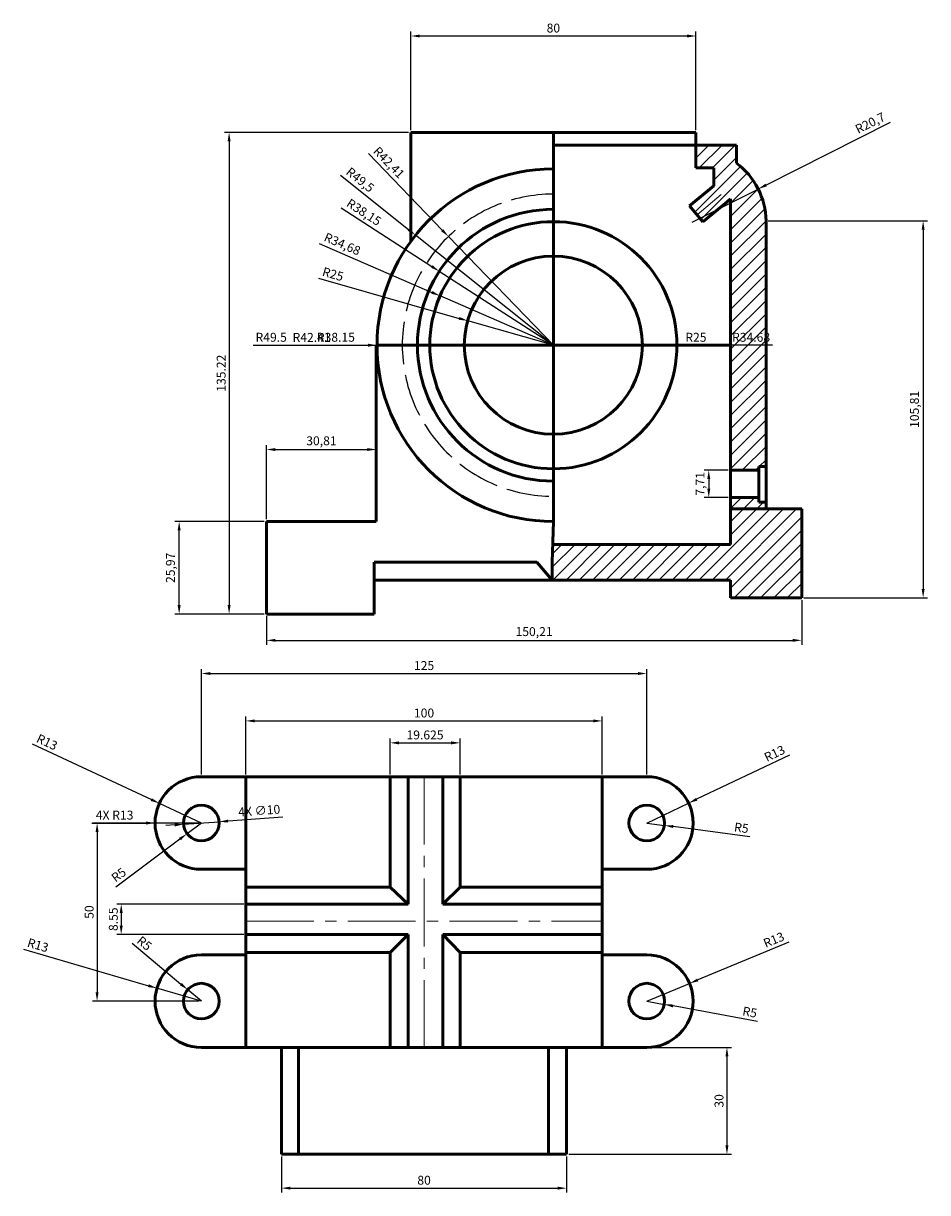
# Model space of a CAD drawing. Units: millimetres. Extents: x 1140 to 1880, y 1480 to 1815.
# Tile 3 of 3: x 1626 to 1880, y 1487 to 1815. Entities that reach past the tile are written whole.
import ezdxf

# ---------------------------------------------------------------- set-up
doc = ezdxf.new("R2010")
doc.units = ezdxf.units.MM
doc.linetypes.add('ACAD_ISO02W100', pattern=[15, 12, -3])
doc.linetypes.add('CENTER2', pattern=[28.575, 19.05, -3.175, 3.175, -3.175])
for name, color, linetype, lineweight in [('M-CNTR', 1, 'CENTER2', 18), ('M-DIMS', 2, 'Continuous', 25), ('M-HATC', 8, 'Continuous', 18), ('M-HIDN', 6, 'ACAD_ISO02W100', 25), ('M-OUTL', 7, 'Continuous', 50)]:
    doc.layers.add(name, color=color, linetype=linetype, lineweight=lineweight)
doc.styles.get("Standard").update_dxf_attribs({"font": 'arial.ttf'})
doc.dimstyles.new('ISO-25', dxfattribs={"dimtxt": 2.5, "dimasz": 2.5, "dimexe": 1.25, "dimexo": 0.625, "dimtad": 1, "dimtxsty": 'Standard', "dimcen": 2.5, "dimadec": 0, "dimazin": 0, "dimtfac": 1, "dimtmove": 0, "dimatfit": 3, "dimfxl": 1, "dimarcsym": 0})

# ---------------------------------------------------------------- blocks, each defined once
blk = doc.blocks.new('*D58')
at = {"layer": 'Defpoints', "color": 0, "transparency": 16777216}
for p in [(1788.55, 1619.58), (1688.55, 1603.92), (1788.55, 1603.92)]:
    blk.add_point(p, dxfattribs=at)
at = {"layer": 'M-DIMS', "color": 0, "lineweight": -2, "transparency": 16777216}
for p, q in [((1688.55, 1604.54), (1688.55, 1620.83)), ((1691.05, 1619.58), (1786.05, 1619.58)), ((1788.55, 1604.54), (1788.55, 1620.83))]:
    blk.add_line(p, q, dxfattribs=at)
at = {"layer": 'M-DIMS', "color": 0, "transparency": 16777216}
for points in [[(1691.05, 1620), (1691.05, 1619.16), (1688.55, 1619.58)], [(1786.05, 1620), (1786.05, 1619.16), (1788.55, 1619.58)]]:
    blk.add_solid(points, dxfattribs=at)
at = {"layer": 'M-DIMS', "color": 0, "transparency": 16777216, "insert": (1738.55, 1621.48), "char_height": 2.5, "attachment_point": 5}
blk.add_mtext('100', dxfattribs=at)
blk = doc.blocks.new('*D59')
at = {"layer": 'Defpoints', "color": 0, "transparency": 16777216}
for p in [(1801.05, 1632.89), (1676.05, 1603.92), (1801.05, 1603.92)]:
    blk.add_point(p, dxfattribs=at)
at = {"layer": 'M-DIMS', "color": 0, "lineweight": -2, "transparency": 16777216}
for p, q in [((1676.05, 1604.54), (1676.05, 1634.14)), ((1678.55, 1632.89), (1798.55, 1632.89)), ((1801.05, 1604.54), (1801.05, 1634.14))]:
    blk.add_line(p, q, dxfattribs=at)
at = {"layer": 'M-DIMS', "color": 0, "transparency": 16777216}
for points in [[(1678.55, 1633.3), (1678.55, 1632.47), (1676.05, 1632.89)], [(1798.55, 1633.3), (1798.55, 1632.47), (1801.05, 1632.89)]]:
    blk.add_solid(points, dxfattribs=at)
at = {"layer": 'M-DIMS', "color": 0, "transparency": 16777216, "insert": (1738.55, 1634.79), "char_height": 2.5, "attachment_point": 5}
blk.add_mtext('125', dxfattribs=at)
blk = doc.blocks.new('*D60')
at = {"layer": 'Defpoints', "color": 0, "transparency": 16777216}
for p in [(1676.05, 1590.92), (1646.78, 1540.92), (1676.05, 1540.92)]:
    blk.add_point(p, dxfattribs=at)
at = {"layer": 'M-DIMS', "color": 0, "lineweight": -2, "transparency": 16777216}
for p, q in [((1675.42, 1590.92), (1645.53, 1590.92)), ((1646.78, 1588.42), (1646.78, 1543.42)), ((1675.42, 1540.92), (1645.53, 1540.92))]:
    blk.add_line(p, q, dxfattribs=at)
at = {"layer": 'M-DIMS', "color": 0, "transparency": 16777216}
for points in [[(1646.36, 1588.42), (1647.19, 1588.42), (1646.78, 1590.92)], [(1646.36, 1543.42), (1647.19, 1543.42), (1646.78, 1540.92)]]:
    blk.add_solid(points, dxfattribs=at)
at = {"layer": 'M-DIMS', "color": 0, "transparency": 16777216, "insert": (1644.88, 1565.92), "char_height": 2.5, "attachment_point": 5, "rotation": 90}
blk.add_mtext('50', dxfattribs=at)
blk = doc.blocks.new('*D61')
at = {"layer": 'Defpoints', "color": 0, "transparency": 16777216}
for p in [(1812.79, 1596.5), (1801.05, 1590.92)]:
    blk.add_point(p, dxfattribs=at)
at = {"layer": 'M-DIMS', "color": 0, "lineweight": -2, "transparency": 16777216}
for p, q in [((1841.13, 1609.99), (1815.05, 1597.58)), ((1801.05, 1590.92), (1812.79, 1596.5))]:
    blk.add_line(p, q, dxfattribs=at)
at = {"layer": 'M-DIMS', "color": 0, "transparency": 16777216}
blk.add_solid([(1814.87, 1597.95), (1815.22, 1597.2), (1812.79, 1596.5)], dxfattribs=at)
at = {"layer": 'M-DIMS', "color": 0, "transparency": 16777216, "insert": (1837.05, 1610.16), "char_height": 2.5, "attachment_point": 5, "rotation": 25.4449}
blk.add_mtext('R13', dxfattribs=at)
blk = doc.blocks.new('*D62')
at = {"layer": 'Defpoints', "color": 0, "transparency": 16777216}
for p in [(1813.05, 1545.91), (1801.05, 1540.92)]:
    blk.add_point(p, dxfattribs=at)
at = {"layer": 'M-DIMS', "color": 0, "lineweight": -2, "transparency": 16777216}
for p, q in [((1840.89, 1557.47), (1815.36, 1546.87)), ((1801.05, 1540.92), (1813.05, 1545.91))]:
    blk.add_line(p, q, dxfattribs=at)
at = {"layer": 'M-DIMS', "color": 0, "transparency": 16777216}
blk.add_solid([(1815.2, 1547.25), (1815.52, 1546.48), (1813.05, 1545.91)], dxfattribs=at)
at = {"layer": 'M-DIMS', "color": 0, "transparency": 16777216, "insert": (1836.82, 1557.84), "char_height": 2.5, "attachment_point": 5, "rotation": 22.5655}
blk.add_mtext('R13', dxfattribs=at)
blk = doc.blocks.new('*D63')
at = {"layer": 'Defpoints', "color": 0, "transparency": 16777216}
for p in [(1663.57, 1544.56), (1676.05, 1540.92)]:
    blk.add_point(p, dxfattribs=at)
at = {"layer": 'M-DIMS', "color": 0, "lineweight": -2, "transparency": 16777216}
for p, q in [((1626.09, 1555.5), (1661.17, 1545.26)), ((1676.05, 1540.92), (1663.57, 1544.56))]:
    blk.add_line(p, q, dxfattribs=at)
at = {"layer": 'M-DIMS', "color": 0, "transparency": 16777216}
blk.add_solid([(1661.29, 1545.66), (1661.05, 1544.86), (1663.57, 1544.56)], dxfattribs=at)
at = {"layer": 'M-DIMS', "color": 0, "transparency": 16777216, "insert": (1630.09, 1556.32), "char_height": 2.5, "attachment_point": 5, "rotation": 343.7247}
blk.add_mtext('R13', dxfattribs=at)
blk = doc.blocks.new('*D64')
at = {"layer": 'Defpoints', "color": 0, "transparency": 16777216}
for p in [(1664.28, 1596.43), (1676.05, 1590.92)]:
    blk.add_point(p, dxfattribs=at)
at = {"layer": 'M-DIMS', "color": 0, "lineweight": -2, "transparency": 16777216}
for p, q in [((1628.53, 1613.16), (1662.01, 1597.49)), ((1676.05, 1590.92), (1664.28, 1596.43))]:
    blk.add_line(p, q, dxfattribs=at)
at = {"layer": 'M-DIMS', "color": 0, "transparency": 16777216}
blk.add_solid([(1662.19, 1597.87), (1661.83, 1597.11), (1664.28, 1596.43)], dxfattribs=at)
at = {"layer": 'M-DIMS', "color": 0, "transparency": 16777216, "insert": (1632.6, 1613.35), "char_height": 2.5, "attachment_point": 5, "rotation": 334.9186}
blk.add_mtext('R13', dxfattribs=at)
blk = doc.blocks.new('*D65')
at = {"layer": 'Defpoints', "color": 0, "transparency": 16777216}
for p in [(1676.05, 1590.92), (1672.04, 1587.93)]:
    blk.add_point(p, dxfattribs=at)
at = {"layer": 'M-DIMS', "color": 0, "lineweight": -2, "transparency": 16777216}
for p, q in [((1676.05, 1590.92), (1672.04, 1587.93)), ((1652.04, 1573.02), (1670.04, 1586.44))]:
    blk.add_line(p, q, dxfattribs=at)
at = {"layer": 'M-DIMS', "color": 0, "transparency": 16777216}
blk.add_solid([(1669.79, 1586.77), (1670.29, 1586.1), (1672.04, 1587.93)], dxfattribs=at)
at = {"layer": 'M-DIMS', "color": 0, "transparency": 16777216, "insert": (1653.03, 1576.12), "char_height": 2.5, "attachment_point": 5, "rotation": 36.7054}
blk.add_mtext('R5', dxfattribs=at)
blk = doc.blocks.new('*D66')
at = {"layer": 'Defpoints', "color": 0, "transparency": 16777216}
for p in [(1672.21, 1544.12), (1676.05, 1540.92)]:
    blk.add_point(p, dxfattribs=at)
at = {"layer": 'M-DIMS', "color": 0, "lineweight": -2, "transparency": 16777216}
for p, q in [((1656.6, 1557.15), (1670.29, 1545.72)), ((1676.05, 1540.92), (1672.21, 1544.12))]:
    blk.add_line(p, q, dxfattribs=at)
at = {"layer": 'M-DIMS', "color": 0, "transparency": 16777216}
blk.add_solid([(1670.56, 1546.04), (1670.02, 1545.4), (1672.21, 1544.12)], dxfattribs=at)
at = {"layer": 'M-DIMS', "color": 0, "transparency": 16777216, "insert": (1659.85, 1556.9), "char_height": 2.5, "attachment_point": 5, "rotation": 320.1593}
blk.add_mtext('R5', dxfattribs=at)
blk = doc.blocks.new('*D67')
at = {"layer": 'Defpoints', "color": 0, "transparency": 16777216}
for p in [(1801.05, 1590.92), (1806, 1590.25)]:
    blk.add_point(p, dxfattribs=at)
at = {"layer": 'M-DIMS', "color": 0, "lineweight": -2, "transparency": 16777216}
for p, q in [((1801.05, 1590.92), (1806, 1590.25)), ((1829.95, 1587.02), (1808.48, 1589.92))]:
    blk.add_line(p, q, dxfattribs=at)
at = {"layer": 'M-DIMS', "color": 0, "transparency": 16777216}
blk.add_solid([(1808.54, 1590.33), (1808.43, 1589.5), (1806, 1590.25)], dxfattribs=at)
at = {"layer": 'M-DIMS', "color": 0, "transparency": 16777216, "insert": (1827.58, 1589.25), "char_height": 2.5, "attachment_point": 5, "rotation": 352.3088}
blk.add_mtext('R5', dxfattribs=at)
blk = doc.blocks.new('*D68')
at = {"layer": 'Defpoints', "color": 0, "transparency": 16777216}
for p in [(1801.05, 1540.92), (1805.97, 1540.01)]:
    blk.add_point(p, dxfattribs=at)
at = {"layer": 'M-DIMS', "color": 0, "lineweight": -2, "transparency": 16777216}
for p, q in [((1801.05, 1540.92), (1805.97, 1540.01)), ((1832.17, 1535.18), (1808.42, 1539.56))]:
    blk.add_line(p, q, dxfattribs=at)
at = {"layer": 'M-DIMS', "color": 0, "transparency": 16777216}
blk.add_solid([(1808.5, 1539.97), (1808.35, 1539.15), (1805.97, 1540.01)], dxfattribs=at)
at = {"layer": 'M-DIMS', "color": 0, "transparency": 16777216, "insert": (1829.91, 1537.52), "char_height": 2.5, "attachment_point": 5, "rotation": 349.5456}
blk.add_mtext('R5', dxfattribs=at)
blk = doc.blocks.new('*D69')
at = {"layer": 'Defpoints', "color": 0, "transparency": 16777216}
for p in [(1844.54, 1654.13), (1694.33, 1649.58), (1844.54, 1642.2)]:
    blk.add_point(p, dxfattribs=at)
at = {"layer": 'M-DIMS', "color": 0, "lineweight": -2, "transparency": 16777216}
for p, q in [((1844.54, 1653.5), (1844.54, 1640.95)), ((1694.33, 1648.95), (1694.33, 1640.95)), ((1696.83, 1642.2), (1842.04, 1642.2))]:
    blk.add_line(p, q, dxfattribs=at)
at = {"layer": 'M-DIMS', "color": 0, "transparency": 16777216}
for points in [[(1696.83, 1642.62), (1696.83, 1641.79), (1694.33, 1642.2)], [(1842.04, 1642.62), (1842.04, 1641.79), (1844.54, 1642.2)]]:
    blk.add_solid(points, dxfattribs=at)
at = {"layer": 'M-DIMS', "color": 0, "transparency": 16777216, "insert": (1769.43, 1644.33), "char_height": 2.5, "attachment_point": 5}
blk.add_mtext('150,21', dxfattribs=at)
blk = doc.blocks.new('*D70')
at = {"layer": 'Defpoints', "color": 0, "transparency": 16777216}
for p in [(1669.81, 1675.55), (1694.33, 1675.55), (1694.33, 1649.58)]:
    blk.add_point(p, dxfattribs=at)
at = {"layer": 'M-DIMS', "color": 0, "lineweight": -2, "transparency": 16777216}
for p, q in [((1693.7, 1675.55), (1668.56, 1675.55)), ((1669.81, 1652.08), (1669.81, 1673.05)), ((1693.7, 1649.58), (1668.56, 1649.58))]:
    blk.add_line(p, q, dxfattribs=at)
at = {"layer": 'M-DIMS', "color": 0, "transparency": 16777216}
for points in [[(1669.39, 1673.05), (1670.22, 1673.05), (1669.81, 1675.55)], [(1669.39, 1652.08), (1670.22, 1652.08), (1669.81, 1649.58)]]:
    blk.add_solid(points, dxfattribs=at)
at = {"layer": 'M-DIMS', "color": 0, "transparency": 16777216, "insert": (1667.68, 1662.56), "char_height": 2.5, "attachment_point": 5, "rotation": 90}
blk.add_mtext('25,97', dxfattribs=at)
blk = doc.blocks.new('*D71')
at = {"layer": 'Defpoints', "color": 0, "transparency": 16777216}
for p in [(1725.14, 1695.77), (1694.33, 1675.55), (1725.14, 1675.55)]:
    blk.add_point(p, dxfattribs=at)
at = {"layer": 'M-DIMS', "color": 0, "lineweight": -2, "transparency": 16777216}
for p, q in [((1694.33, 1676.17), (1694.33, 1697.02)), ((1725.14, 1676.17), (1725.14, 1697.02)), ((1696.83, 1695.77), (1722.64, 1695.77))]:
    blk.add_line(p, q, dxfattribs=at)
at = {"layer": 'M-DIMS', "color": 0, "transparency": 16777216}
for points in [[(1696.83, 1696.18), (1696.83, 1695.35), (1694.33, 1695.77)], [(1722.64, 1696.18), (1722.64, 1695.35), (1725.14, 1695.77)]]:
    blk.add_solid(points, dxfattribs=at)
at = {"layer": 'M-DIMS', "color": 0, "transparency": 16777216, "insert": (1709.74, 1697.89), "char_height": 2.5, "attachment_point": 5}
blk.add_mtext('30,81', dxfattribs=at)
blk = doc.blocks.new('*D72')
at = {"layer": 'Defpoints', "color": 0, "transparency": 16777216}
for p in [(1814.84, 1811.85), (1734.84, 1784.8), (1814.84, 1784.8)]:
    blk.add_point(p, dxfattribs=at)
at = {"layer": 'M-DIMS', "color": 0, "lineweight": -2, "transparency": 16777216}
for p, q in [((1734.84, 1785.42), (1734.84, 1813.1)), ((1737.34, 1811.85), (1812.34, 1811.85)), ((1814.84, 1785.42), (1814.84, 1813.1))]:
    blk.add_line(p, q, dxfattribs=at)
at = {"layer": 'M-DIMS', "color": 0, "transparency": 16777216}
for points in [[(1737.34, 1812.26), (1737.34, 1811.43), (1734.84, 1811.85)], [(1812.34, 1812.26), (1812.34, 1811.43), (1814.84, 1811.85)]]:
    blk.add_solid(points, dxfattribs=at)
at = {"layer": 'M-DIMS', "color": 0, "transparency": 16777216, "insert": (1774.84, 1813.75), "char_height": 2.5, "attachment_point": 5}
blk.add_mtext('80', dxfattribs=at)
blk = doc.blocks.new('*D73')
at = {"layer": 'Defpoints', "color": 0, "transparency": 16777216}
for p in [(1834.52, 1759.94), (1844.54, 1654.13), (1878.62, 1654.13)]:
    blk.add_point(p, dxfattribs=at)
at = {"layer": 'M-DIMS', "color": 0, "lineweight": -2, "transparency": 16777216}
for p, q in [((1835.15, 1759.94), (1879.87, 1759.94)), ((1878.62, 1757.44), (1878.62, 1656.63)), ((1845.16, 1654.13), (1879.87, 1654.13))]:
    blk.add_line(p, q, dxfattribs=at)
at = {"layer": 'M-DIMS', "color": 0, "transparency": 16777216}
for points in [[(1878.2, 1757.44), (1879.04, 1757.44), (1878.62, 1759.94)], [(1878.2, 1656.63), (1879.04, 1656.63), (1878.62, 1654.13)]]:
    blk.add_solid(points, dxfattribs=at)
at = {"layer": 'M-DIMS', "color": 0, "transparency": 16777216, "insert": (1876.49, 1707.03), "char_height": 2.5, "attachment_point": 5, "rotation": 90}
blk.add_mtext('105,81', dxfattribs=at)
blk = doc.blocks.new('*D74')
at = {"layer": 'Defpoints', "color": 0, "transparency": 16777216}
for p in [(1832.32, 1768.89), (1813.83, 1759.59)]:
    blk.add_point(p, dxfattribs=at)
at = {"layer": 'M-DIMS', "color": 0, "lineweight": -2, "transparency": 16777216}
for p, q in [((1869.36, 1787.53), (1834.55, 1770.01)), ((1813.83, 1759.59), (1832.32, 1768.89))]:
    blk.add_line(p, q, dxfattribs=at)
at = {"layer": 'M-DIMS', "color": 0, "transparency": 16777216}
blk.add_solid([(1834.36, 1770.39), (1834.74, 1769.64), (1832.32, 1768.89)], dxfattribs=at)
at = {"layer": 'M-DIMS', "color": 0, "transparency": 16777216, "insert": (1863.88, 1787.15), "char_height": 2.5, "attachment_point": 5, "rotation": 26.7111}
blk.add_mtext('R20,7', dxfattribs=at)
blk = doc.blocks.new('*D75')
at = {"layer": 'Defpoints', "color": 0, "transparency": 16777216}
for p in [(1736.16, 1755.94), (1774.84, 1725.05)]:
    blk.add_point(p, dxfattribs=at)
at = {"layer": 'M-DIMS', "color": 0, "lineweight": -2, "transparency": 16777216}
for p, q in [((1715.11, 1772.75), (1734.21, 1757.5)), ((1774.84, 1725.05), (1736.16, 1755.94))]:
    blk.add_line(p, q, dxfattribs=at)
at = {"layer": 'M-DIMS', "color": 0, "transparency": 16777216}
blk.add_solid([(1734.47, 1757.82), (1733.95, 1757.17), (1736.16, 1755.94)], dxfattribs=at)
at = {"layer": 'M-DIMS', "color": 0, "transparency": 16777216, "insert": (1720.41, 1771.24), "char_height": 2.5, "attachment_point": 5, "rotation": 321.3853}
blk.add_mtext('R49,5', dxfattribs=at)
blk = doc.blocks.new('*D76')
at = {"layer": 'Defpoints', "color": 0, "transparency": 16777216}
for p in [(1745.38, 1755.55), (1774.84, 1725.05)]:
    blk.add_point(p, dxfattribs=at)
at = {"layer": 'M-DIMS', "color": 0, "lineweight": -2, "transparency": 16777216}
for p, q in [((1722.91, 1778.82), (1743.64, 1757.35)), ((1774.84, 1725.05), (1745.38, 1755.55))]:
    blk.add_line(p, q, dxfattribs=at)
at = {"layer": 'M-DIMS', "color": 0, "transparency": 16777216}
blk.add_solid([(1743.94, 1757.64), (1743.34, 1757.06), (1745.38, 1755.55)], dxfattribs=at)
at = {"layer": 'M-DIMS', "color": 0, "transparency": 16777216, "insert": (1728.47, 1776.12), "char_height": 2.5, "attachment_point": 5, "rotation": 314.0026}
blk.add_mtext('R42,41', dxfattribs=at)
blk = doc.blocks.new('*D77')
at = {"layer": 'Defpoints', "color": 0, "transparency": 16777216}
for p in [(1742.82, 1745.78), (1774.84, 1725.05)]:
    blk.add_point(p, dxfattribs=at)
at = {"layer": 'M-DIMS', "color": 0, "lineweight": -2, "transparency": 16777216}
for p, q in [((1715.27, 1763.63), (1740.72, 1747.14)), ((1774.84, 1725.05), (1742.82, 1745.78))]:
    blk.add_line(p, q, dxfattribs=at)
at = {"layer": 'M-DIMS', "color": 0, "transparency": 16777216}
blk.add_solid([(1740.95, 1747.49), (1740.5, 1746.79), (1742.82, 1745.78)], dxfattribs=at)
at = {"layer": 'M-DIMS', "color": 0, "transparency": 16777216, "insert": (1721.5, 1762.12), "char_height": 2.5, "attachment_point": 5, "rotation": 327.07}
blk.add_mtext('R38,15', dxfattribs=at)
blk = doc.blocks.new('*D78')
at = {"layer": 'Defpoints', "color": 0, "transparency": 16777216}
for p in [(1743.04, 1738.88), (1774.84, 1725.05)]:
    blk.add_point(p, dxfattribs=at)
at = {"layer": 'M-DIMS', "color": 0, "lineweight": -2, "transparency": 16777216}
for p, q in [((1709.11, 1753.63), (1740.74, 1739.87)), ((1774.84, 1725.05), (1743.04, 1738.88))]:
    blk.add_line(p, q, dxfattribs=at)
at = {"layer": 'M-DIMS', "color": 0, "transparency": 16777216}
blk.add_solid([(1740.91, 1740.25), (1740.58, 1739.49), (1743.04, 1738.88)], dxfattribs=at)
at = {"layer": 'M-DIMS', "color": 0, "transparency": 16777216, "insert": (1715.49, 1753.17), "char_height": 2.5, "attachment_point": 5, "rotation": 336.4971}
blk.add_mtext('R34,68', dxfattribs=at)
blk = doc.blocks.new('*D79')
at = {"layer": 'Defpoints', "color": 0, "transparency": 16777216}
for p in [(1750.8, 1731.9), (1774.84, 1725.05)]:
    blk.add_point(p, dxfattribs=at)
at = {"layer": 'M-DIMS', "color": 0, "lineweight": -2, "transparency": 16777216}
for p, q in [((1708.88, 1743.86), (1748.4, 1732.59)), ((1774.84, 1725.05), (1750.8, 1731.9))]:
    blk.add_line(p, q, dxfattribs=at)
at = {"layer": 'M-DIMS', "color": 0, "transparency": 16777216}
blk.add_solid([(1748.51, 1732.99), (1748.28, 1732.19), (1750.8, 1731.9)], dxfattribs=at)
at = {"layer": 'M-DIMS', "color": 0, "transparency": 16777216, "insert": (1712.89, 1744.69), "char_height": 2.5, "attachment_point": 5, "rotation": 344.0796}
blk.add_mtext('R25', dxfattribs=at)
blk = doc.blocks.new('*D80')
at = {"layer": 'Defpoints', "color": 0, "transparency": 16777216}
for p in [(1824.54, 1689.98), (1818.45, 1682.27), (1824.54, 1682.27)]:
    blk.add_point(p, dxfattribs=at)
at = {"layer": 'M-DIMS', "color": 0, "lineweight": -2, "transparency": 16777216}
for p, q in [((1823.91, 1689.98), (1817.2, 1689.98)), ((1818.45, 1687.48), (1818.45, 1684.77)), ((1823.91, 1682.27), (1817.2, 1682.27))]:
    blk.add_line(p, q, dxfattribs=at)
at = {"layer": 'M-DIMS', "color": 0, "transparency": 16777216}
for points in [[(1818.03, 1687.48), (1818.87, 1687.48), (1818.45, 1689.98)], [(1818.03, 1684.77), (1818.87, 1684.77), (1818.45, 1682.27)]]:
    blk.add_solid(points, dxfattribs=at)
at = {"layer": 'M-DIMS', "color": 0, "transparency": 16777216, "insert": (1816.32, 1686.13), "char_height": 2.5, "attachment_point": 5, "rotation": 90}
blk.add_mtext('7,71', dxfattribs=at)
blk = doc.blocks.new('HOLE-D10')
blk.add_circle((5, 5), 5)
blk = doc.blocks.new('*D87')
at = {"layer": 'Defpoints', "color": 0, "transparency": 16777216}
for p in [(1734.84, 1784.8), (1683.83, 1649.58), (1694.33, 1649.58)]:
    blk.add_point(p, dxfattribs=at)
at = {"layer": 'M-DIMS', "color": 0, "lineweight": -2, "transparency": 16777216}
for p, q in [((1734.22, 1784.8), (1682.58, 1784.8)), ((1683.83, 1782.3), (1683.83, 1652.08)), ((1693.7, 1649.58), (1682.58, 1649.58))]:
    blk.add_line(p, q, dxfattribs=at)
at = {"layer": 'M-DIMS', "color": 0, "transparency": 16777216}
for points in [[(1683.41, 1782.3), (1684.25, 1782.3), (1683.83, 1784.8)], [(1683.41, 1652.08), (1684.25, 1652.08), (1683.83, 1649.58)]]:
    blk.add_solid(points, dxfattribs=at)
at = {"layer": 'M-DIMS', "color": 0, "transparency": 16777216, "insert": (1681.93, 1717.19), "char_height": 2.5, "attachment_point": 5, "rotation": 90}
blk.add_mtext('135.22', dxfattribs=at)
blk = doc.blocks.new('*D90')
at = {"layer": 'Defpoints', "color": 0, "transparency": 16777216}
for p in [(1748.64, 1613.42), (1729.01, 1603.92), (1748.64, 1603.92)]:
    blk.add_point(p, dxfattribs=at)
at = {"layer": 'M-DIMS', "color": 0, "lineweight": -2, "transparency": 16777216}
for p, q in [((1729.01, 1604.54), (1729.01, 1614.67)), ((1731.51, 1613.42), (1746.14, 1613.42)), ((1748.64, 1604.54), (1748.64, 1614.67))]:
    blk.add_line(p, q, dxfattribs=at)
at = {"layer": 'M-DIMS', "color": 0, "transparency": 16777216}
for points in [[(1731.51, 1613.84), (1731.51, 1613), (1729.01, 1613.42)], [(1746.14, 1613.84), (1746.14, 1613), (1748.64, 1613.42)]]:
    blk.add_solid(points, dxfattribs=at)
at = {"layer": 'M-DIMS', "color": 0, "transparency": 16777216, "insert": (1738.82, 1615.32), "char_height": 2.5, "attachment_point": 5}
blk.add_mtext('19.625', dxfattribs=at)
blk = doc.blocks.new('*D91')
at = {"layer": 'Defpoints', "color": 0, "transparency": 16777216}
for p in [(1688.55, 1568.18), (1653.55, 1559.63), (1688.55, 1559.63)]:
    blk.add_point(p, dxfattribs=at)
at = {"layer": 'M-DIMS', "color": 0, "lineweight": -2, "transparency": 16777216}
for p, q in [((1687.92, 1568.18), (1652.3, 1568.18)), ((1653.55, 1565.68), (1653.55, 1562.13)), ((1687.92, 1559.63), (1652.3, 1559.63))]:
    blk.add_line(p, q, dxfattribs=at)
at = {"layer": 'M-DIMS', "color": 0, "transparency": 16777216}
for points in [[(1653.13, 1565.68), (1653.97, 1565.68), (1653.55, 1568.18)], [(1653.13, 1562.13), (1653.97, 1562.13), (1653.55, 1559.63)]]:
    blk.add_solid(points, dxfattribs=at)
at = {"layer": 'M-DIMS', "color": 0, "transparency": 16777216, "insert": (1651.65, 1563.91), "char_height": 2.5, "attachment_point": 5, "rotation": 90}
blk.add_mtext('8.55', dxfattribs=at)
blk = doc.blocks.new('*D92')
at = {"layer": 'Defpoints', "color": 0, "transparency": 16777216}
for p in [(1698.55, 1497.92), (1778.55, 1497.92), (1778.55, 1488.42)]:
    blk.add_point(p, dxfattribs=at)
at = {"layer": 'M-DIMS', "color": 0, "lineweight": -2, "transparency": 16777216}
for p, q in [((1698.55, 1497.29), (1698.55, 1487.17)), ((1778.55, 1497.29), (1778.55, 1487.17)), ((1701.05, 1488.42), (1776.05, 1488.42))]:
    blk.add_line(p, q, dxfattribs=at)
at = {"layer": 'M-DIMS', "color": 0, "transparency": 16777216}
for points in [[(1701.05, 1488.84), (1701.05, 1488), (1698.55, 1488.42)], [(1776.05, 1488.84), (1776.05, 1488), (1778.55, 1488.42)]]:
    blk.add_solid(points, dxfattribs=at)
at = {"layer": 'M-DIMS', "color": 0, "transparency": 16777216, "insert": (1738.55, 1490.32), "char_height": 2.5, "attachment_point": 5}
blk.add_mtext('80', dxfattribs=at)
blk = doc.blocks.new('*D93')
at = {"layer": 'Defpoints', "color": 0, "transparency": 16777216}
for p in [(1778.55, 1527.92), (1778.55, 1497.92), (1823.55, 1497.92)]:
    blk.add_point(p, dxfattribs=at)
at = {"layer": 'M-DIMS', "color": 0, "lineweight": -2, "transparency": 16777216}
for p, q in [((1779.17, 1527.92), (1824.8, 1527.92)), ((1823.55, 1525.42), (1823.55, 1500.42)), ((1779.17, 1497.92), (1824.8, 1497.92))]:
    blk.add_line(p, q, dxfattribs=at)
at = {"layer": 'M-DIMS', "color": 0, "transparency": 16777216}
for points in [[(1823.13, 1525.42), (1823.97, 1525.42), (1823.55, 1527.92)], [(1823.13, 1500.42), (1823.97, 1500.42), (1823.55, 1497.92)]]:
    blk.add_solid(points, dxfattribs=at)
at = {"layer": 'M-DIMS', "color": 0, "transparency": 16777216, "insert": (1821.65, 1512.92), "char_height": 2.5, "attachment_point": 5, "rotation": 90}
blk.add_mtext('30', dxfattribs=at)
blk = doc.blocks.new('*D98')
at = {"layer": 'Defpoints', "color": 0, "transparency": 16777216}
for p in [(1725.34, 1725.04), (1774.84, 1725.05)]:
    blk.add_point(p, dxfattribs=at)
at = {"layer": 'M-DIMS', "color": 0, "lineweight": -2, "transparency": 16777216}
for p, q in [((1690.56, 1725.04), (1722.84, 1725.04)), ((1774.84, 1725.05), (1725.34, 1725.04))]:
    blk.add_line(p, q, dxfattribs=at)
at = {"layer": 'M-DIMS', "color": 0, "transparency": 16777216}
blk.add_solid([(1722.84, 1725.46), (1722.84, 1724.63), (1725.34, 1725.04)], dxfattribs=at)
at = {"layer": 'M-DIMS', "color": 0, "transparency": 16777216, "insert": (1695.64, 1726.95), "char_height": 2.5, "attachment_point": 5, "rotation": 0.0005}
blk.add_mtext('R49.5', dxfattribs=at)
blk = doc.blocks.new('*D99')
at = {"layer": 'Defpoints', "color": 0, "transparency": 16777216}
for p in [(1732.43, 1725.04), (1774.84, 1725.05)]:
    blk.add_point(p, dxfattribs=at)
at = {"layer": 'M-DIMS', "color": 0, "lineweight": -2, "transparency": 16777216}
for p, q in [((1701.18, 1725.04), (1729.93, 1725.04)), ((1774.84, 1725.05), (1732.43, 1725.04))]:
    blk.add_line(p, q, dxfattribs=at)
at = {"layer": 'M-DIMS', "color": 0, "transparency": 16777216}
blk.add_solid([(1729.93, 1725.46), (1729.93, 1724.63), (1732.43, 1725.04)], dxfattribs=at)
at = {"layer": 'M-DIMS', "color": 0, "transparency": 16777216, "insert": (1706.98, 1726.92), "char_height": 2.5, "attachment_point": 5, "rotation": 0.0005}
blk.add_mtext('R42.41', dxfattribs=at)
blk = doc.blocks.new('*D100')
at = {"layer": 'Defpoints', "color": 0, "transparency": 16777216}
for p in [(1736.69, 1725.04), (1774.84, 1725.05)]:
    blk.add_point(p, dxfattribs=at)
at = {"layer": 'M-DIMS', "color": 0, "lineweight": -2, "transparency": 16777216}
for p, q in [((1707.75, 1725.04), (1734.19, 1725.04)), ((1774.84, 1725.05), (1736.69, 1725.04))]:
    blk.add_line(p, q, dxfattribs=at)
at = {"layer": 'M-DIMS', "color": 0, "transparency": 16777216}
blk.add_solid([(1734.19, 1725.46), (1734.19, 1724.63), (1736.69, 1725.04)], dxfattribs=at)
at = {"layer": 'M-DIMS', "color": 0, "transparency": 16777216, "insert": (1713.8, 1726.95), "char_height": 2.5, "attachment_point": 5, "rotation": 0.0006}
blk.add_mtext('R38.15', dxfattribs=at)
blk = doc.blocks.new('*D101')
at = {"layer": 'Defpoints', "color": 0, "transparency": 16777216}
for p in [(1774.84, 1725.05), (1809.52, 1725.04)]:
    blk.add_point(p, dxfattribs=at)
at = {"layer": 'M-DIMS', "color": 0, "lineweight": -2, "transparency": 16777216}
for p, q in [((1774.84, 1725.05), (1809.52, 1725.04)), ((1836.37, 1725.04), (1812.02, 1725.04))]:
    blk.add_line(p, q, dxfattribs=at)
at = {"layer": 'M-DIMS', "color": 0, "transparency": 16777216}
blk.add_solid([(1812.02, 1725.46), (1812.02, 1724.63), (1809.52, 1725.04)], dxfattribs=at)
at = {"layer": 'M-DIMS', "color": 0, "transparency": 16777216, "insert": (1830.33, 1726.95), "char_height": 2.5, "attachment_point": 5, "rotation": 359.9993}
blk.add_mtext('R34.68', dxfattribs=at)
blk = doc.blocks.new('*D102')
at = {"layer": 'Defpoints', "color": 0, "transparency": 16777216}
for p in [(1774.84, 1725.05), (1799.84, 1725.04)]:
    blk.add_point(p, dxfattribs=at)
at = {"layer": 'M-DIMS', "color": 0, "lineweight": -2, "transparency": 16777216}
for p, q in [((1774.84, 1725.05), (1799.84, 1725.04)), ((1818.46, 1725.04), (1802.34, 1725.04))]:
    blk.add_line(p, q, dxfattribs=at)
at = {"layer": 'M-DIMS', "color": 0, "transparency": 16777216}
blk.add_solid([(1802.34, 1725.46), (1802.34, 1724.63), (1799.84, 1725.04)], dxfattribs=at)
at = {"layer": 'M-DIMS', "color": 0, "transparency": 16777216, "insert": (1814.84, 1726.95), "char_height": 2.5, "attachment_point": 5, "rotation": 359.9991}
blk.add_mtext('R25', dxfattribs=at)
blk = doc.blocks.new('*D104')
at = {"layer": 'Defpoints', "color": 0, "transparency": 16777216}
for p in [(1663.05, 1590.92), (1676.05, 1590.92)]:
    blk.add_point(p, dxfattribs=at)
at = {"layer": 'M-DIMS', "color": 0, "lineweight": -2, "transparency": 16777216}
for p, q in [((1645.35, 1590.92), (1660.55, 1590.92)), ((1676.05, 1590.92), (1663.05, 1590.92))]:
    blk.add_line(p, q, dxfattribs=at)
at = {"layer": 'M-DIMS', "color": 0, "transparency": 16777216}
blk.add_solid([(1660.55, 1591.34), (1660.55, 1590.5), (1663.05, 1590.92)], dxfattribs=at)
at = {"layer": 'M-DIMS', "color": 0, "transparency": 16777216, "insert": (1651.7, 1592.82), "char_height": 2.5, "attachment_point": 5, "rotation": 359.9994}
blk.add_mtext('4X R13', dxfattribs=at)
blk = doc.blocks.new('*D105')
at = {"layer": 'Defpoints', "color": 0, "transparency": 16777216}
for p in [(1671.06, 1590.56), (1681.04, 1591.28)]:
    blk.add_point(p, dxfattribs=at)
at = {"layer": 'M-DIMS', "color": 0, "lineweight": -2, "transparency": 16777216}
for p, q in [((1698.87, 1592.58), (1683.53, 1591.46)), ((1668.57, 1590.38), (1666.08, 1590.19)), ((1671.06, 1590.56), (1681.04, 1591.28))]:
    blk.add_line(p, q, dxfattribs=at)
at = {"layer": 'M-DIMS', "color": 0, "transparency": 16777216}
for points in [[(1683.5, 1591.88), (1683.56, 1591.05), (1681.04, 1591.28)], [(1668.54, 1590.79), (1668.6, 1589.96), (1671.06, 1590.56)]]:
    blk.add_solid(points, dxfattribs=at)
at = {"layer": 'M-DIMS', "color": 0, "transparency": 16777216, "insert": (1692.3, 1594.08), "char_height": 2.5, "attachment_point": 5, "rotation": 4.1517}
blk.add_mtext('4X ∅10', dxfattribs=at)

msp = doc.modelspace()

# ---------------------------------------------------------------- hatches: boundary and pattern name
at = {"layer": 'M-HATC'}
h = msp.add_hatch(dxfattribs=at)
h.set_pattern_fill('ANSI31', color=256, scale=0.83)
h.paths.add_polyline_path([(1844.5379, 1679.1293), (1824.5379, 1679.1293), (1824.5379, 1669.1293), (1774.6703, 1669.1293), (1774.5379, 1664.1293), (1774.5379, 1659.1293), (1824.5379, 1659.1293), (1824.5379, 1654.1293), (1844.5379, 1654.1293)])
h.paths.add_polyline_path([(1834.5221, 1759.9406, 0.23234266), (1826.1977, 1776.1821), (1826.1977, 1781.1821), (1814.8403, 1781.1821), (1814.8403, 1774.7988), (1819.8403, 1774.7988), (1819.8403, 1769.7988), (1813.0831, 1764.171), (1816.8285, 1759.6738), (1823.5858, 1765.3016), (1824.5379, 1766.1046), (1824.5379, 1759.9406), (1824.5379, 1689.9787), (1832.5221, 1689.9787), (1832.5221, 1690.9837), (1834.5221, 1690.9837)])
h.paths.add_polyline_path([(1834.5221, 1680.9837), (1832.5221, 1680.9837), (1832.5221, 1682.2732), (1824.5379, 1682.2732), (1824.5379, 1679.1293), (1834.5221, 1679.1293)])

# ---------------------------------------------------------------- linework, layer by layer
at = {"layer": 'M-CNTR'}
for p, q in [((1821.9061, 1767.3184), (1815.1488, 1761.6907)), ((1738.5495, 1603.9189), (1738.5495, 1527.9189)), ((1688.5495, 1563.3802), (1788.5495, 1563.3802))]:
    msp.add_line(p, q, dxfattribs=at)
at = {"layer": 'M-HIDN'}
for radius in [49.5, 42.4113]:
    msp.add_arc((1774.8403, 1725.0454), radius, 90, 270, dxfattribs=at)
at = {"layer": 'M-OUTL'}
for p, q in [((1774.8403, 1784.7988), (1734.8403, 1784.7988)), ((1734.8403, 1784.7988), (1734.8403, 1754.2044)), ((1774.8403, 1725.0454), (1774.8403, 1784.7988)), ((1774.8403, 1784.7988), (1814.8403, 1784.7988)), ((1814.8403, 1784.7988), (1814.8403, 1774.7988)), ((1826.1977, 1781.1821), (1774.8403, 1781.1821)), ((1826.1977, 1776.1821), (1826.1977, 1781.1821)), ((1814.8403, 1774.7988), (1819.8403, 1774.7988)), ((1819.8403, 1774.7988), (1819.8403, 1769.7988)), ((1819.8403, 1769.7988), (1813.0831, 1764.171)), ((1823.5858, 1765.3016), (1824.5379, 1766.1046)), ((1824.5379, 1759.9406), (1824.5379, 1766.1046)), ((1813.0831, 1764.171), (1816.8285, 1759.6738)), ((1823.5858, 1765.3016), (1816.8285, 1759.6738)), ((1824.5379, 1679.1293), (1824.5379, 1759.9406)), ((1834.5221, 1679.1293), (1834.5221, 1759.9406)), ((1725.1427, 1675.5454), (1725.1427, 1725.0454)), ((1725.1427, 1725.0454), (1824.5379, 1725.0454)), ((1774.8403, 1725.0454), (1774.8403, 1675.5454)), ((1834.5221, 1690.9837), (1832.5221, 1690.9837)), ((1832.5221, 1690.9837), (1832.5221, 1680.9837)), ((1834.5221, 1685.9837), (1834.5221, 1690.9837)), ((1824.5379, 1689.9787), (1832.5221, 1689.9787)), ((1824.5379, 1682.2732), (1832.5221, 1682.2732)), ((1832.5221, 1680.9837), (1834.5221, 1680.9837)), ((1844.5379, 1679.1293), (1824.5379, 1679.1293)), ((1824.5379, 1679.1293), (1824.5379, 1669.1293)), ((1844.5379, 1654.1293), (1844.5379, 1679.1293)), ((1694.3292, 1649.5795), (1694.3292, 1675.5454)), ((1694.3292, 1675.5454), (1725.1427, 1675.5454)), ((1774.8403, 1675.5454), (1774.5379, 1664.1293)), ((1824.5379, 1669.1293), (1774.6703, 1669.1293)), ((1724.5379, 1649.5795), (1724.5379, 1664.1293)), ((1724.5379, 1664.1293), (1770.1892, 1664.1293)), ((1724.5379, 1664.1293), (1724.5379, 1659.1293)), ((1774.5379, 1659.1293), (1770.1892, 1664.1293)), ((1774.5379, 1664.1293), (1774.5379, 1659.1293)), ((1724.5379, 1659.1293), (1774.5379, 1659.1293)), ((1774.5379, 1659.1293), (1824.5379, 1659.1293)), ((1824.5379, 1659.1293), (1824.5379, 1654.1293)), ((1824.5379, 1654.1293), (1844.5379, 1654.1293)), ((1694.3292, 1649.5795), (1724.5379, 1649.5795)), ((1676.0495, 1603.9189), (1801.0495, 1603.9189)), ((1738.5495, 1603.9189), (1688.5495, 1603.9189)), ((1688.5495, 1603.9189), (1688.5495, 1527.9189)), ((1729.0103, 1603.9189), (1729.0103, 1572.9366)), ((1734.0515, 1603.9189), (1734.0515, 1568.1835)), ((1743.8229, 1603.9189), (1743.8229, 1568.1835)), ((1748.6351, 1603.9189), (1748.6351, 1572.9366)), ((1788.5495, 1527.9189), (1788.5495, 1603.9189)), ((1676.0495, 1577.9189), (1688.5495, 1577.9189)), ((1801.0495, 1577.9189), (1788.5495, 1577.9189)), ((1688.5495, 1572.9366), (1729.0103, 1572.9366)), ((1729.0103, 1572.9366), (1734.0515, 1568.1835)), ((1748.6351, 1572.9366), (1743.8229, 1568.1835)), ((1748.6351, 1572.9366), (1788.5495, 1572.9366)), ((1688.5495, 1568.1835), (1734.0515, 1568.1835)), ((1743.8229, 1568.1835), (1788.5495, 1568.1835)), ((1688.5495, 1559.6326), (1734.0515, 1559.6326)), ((1729.0103, 1554.6127), (1734.0515, 1559.6326)), ((1734.0515, 1559.6326), (1734.0515, 1527.9189)), ((1743.8229, 1559.6326), (1788.5495, 1559.6326)), ((1743.8229, 1559.6326), (1743.8229, 1527.9189)), ((1743.8229, 1559.6326), (1748.6351, 1554.6127)), ((1676.0495, 1553.9189), (1688.5495, 1553.9189)), ((1688.5495, 1554.6127), (1729.0103, 1554.6127)), ((1729.0103, 1554.6127), (1729.0103, 1527.9189)), ((1748.6351, 1554.6127), (1788.5495, 1554.6127)), ((1748.6351, 1554.6127), (1748.6351, 1527.9189)), ((1801.0495, 1553.9189), (1788.5495, 1553.9189)), ((1801.0495, 1527.9189), (1676.0495, 1527.9189)), ((1738.5495, 1527.9189), (1698.5495, 1527.9189)), ((1698.5495, 1527.9189), (1698.5495, 1497.9189)), ((1703.3141, 1527.9189), (1703.3141, 1497.9189)), ((1773.491, 1497.9189), (1773.491, 1527.9189)), ((1778.5495, 1497.9189), (1778.5495, 1527.9189)), ((1698.5495, 1497.9189), (1778.5495, 1497.9189))]:
    msp.add_line(p, q, dxfattribs=at)
for radius in [34.68, 25]:
    msp.add_circle((1774.8403, 1725.0454), radius, dxfattribs=at)
for centre, radius, start, end in [((1813.8275, 1759.5878), 20.6977, 0.976585, 53.297304), ((1774.8403, 1725.0454), 49.5, 90, 270), ((1774.8403, 1725.0454), 38.1493, 90, 270), ((1676.0495, 1590.9189), 13, 90, 270), ((1801.0495, 1590.9189), 13, 270, 90), ((1676.0495, 1540.9189), 13, 90, 270), ((1801.0495, 1540.9189), 13, 270, 90)]:
    msp.add_arc(centre, radius, start, end, dxfattribs=at)

# ---------------------------------------------------------------- block references
for p in [(1671.049, 1585.919), (1796.049, 1585.919), (1671.049, 1535.919), (1796.049, 1535.919)]:
    msp.add_blockref('HOLE-D10', p, dxfattribs=at)

# ---------------------------------------------------------------- dimensions: what is measured, and where the dimension line sits
at = {"layer": 'M-DIMS'}
for base, p1, p2, override, picture, middle in [((1814.8403, 1811.8461), (1734.8403, 1784.7988), (1814.8403, 1784.7988), {"dimclrd": 0, "dimclre": 0, "dimclrt": 0}, '*D72', (1774.8403, 1813.7476)), ((1725.1427, 1695.7669), (1694.3292, 1675.5454), (1725.1427, 1675.5454), {"dimclrd": 0, "dimclre": 0, "dimclrt": 0}, '*D71', (1709.736, 1697.8943)), ((1844.5379, 1642.2022), (1694.3292, 1649.5795), (1844.5379, 1654.1293), {"dimclrd": 0, "dimclre": 0, "dimclrt": 0}, '*D69', (1769.4335, 1644.3296)), ((1801.0495, 1632.8878), (1676.0495, 1603.9189), (1801.0495, 1603.9189), {"dimclrd": 0, "dimclre": 0, "dimclrt": 0}, '*D59', (1738.5495, 1634.7893)), ((1788.5495, 1619.5802), (1688.5495, 1603.9189), (1788.5495, 1603.9189), {"dimclrd": 0, "dimclre": 0, "dimclrt": 0}, '*D58', (1738.5495, 1621.4816)), ((1748.6351, 1613.4189), (1729.0103, 1603.9189), (1748.6351, 1603.9189), {"dimdec": 3, "dimlfac": 1, "dimrnd": 0, "dimzin": 0, "dimdsep": 46, "dimlunit": 2}, '*D90', (1738.8227, 1615.3203)), ((1778.5495, 1488.4189), (1698.5495, 1497.9189), (1778.5495, 1497.9189), {"dimdec": 0, "dimlfac": 1, "dimrnd": 0, "dimzin": 0, "dimdsep": 46, "dimlunit": 2}, '*D92', (1738.5495, 1490.3203))]:
    dim = msp.add_linear_dim(base=base, p1=p1, p2=p2, dimstyle='ISO-25', override=override, dxfattribs=at)
    dim.commit()
    dim.dimension.update_dxf_attribs({"geometry": picture, "text_midpoint": middle})
for center, mpoint, override, picture, middle in [((1813.8275, 1759.5878), (1832.3164, 1768.8912), {"dimclrd": 0, "dimclre": 0, "dimclrt": 0}, '*D74', (1864.832, 1785.2528)), ((1774.8403, 1725.0454), (1745.3775, 1755.5522), {"dimclrd": 0, "dimclre": 0, "dimclrt": 0}, '*D76', (1726.9379, 1774.6452)), ((1774.8403, 1725.0454), (1736.163, 1755.9374), {"dimclrd": 0, "dimclre": 0, "dimclrt": 0}, '*D75', (1719.0812, 1769.5808)), ((1774.8403, 1725.0454), (1742.8203, 1745.7839), {"dimclrd": 0, "dimclre": 0, "dimclrt": 0}, '*D77', (1720.3484, 1760.3382)), ((1774.8403, 1725.0454), (1743.0374, 1738.8756), {"dimclrd": 0, "dimclre": 0, "dimclrt": 0}, '*D78', (1714.646, 1751.2223)), ((1774.8403, 1725.0454), (1750.7992, 1731.9029), {"dimclrd": 0, "dimclre": 0, "dimclrt": 0}, '*D79', (1712.365, 1742.866)), ((1774.8403, 1725.0454), (1725.3403, 1725.045), {"dimdec": 1, "dimlfac": 1, "dimrnd": 0, "dimzin": 0, "dimdsep": 46, "dimlunit": 2}, '*D98', (1695.6403, 1725.0448)), ((1774.8403, 1725.0454), (1732.429, 1725.045), {"dimdec": 2, "dimlfac": 1, "dimrnd": 0, "dimzin": 0, "dimdsep": 46, "dimlunit": 2}, '*D99', (1706.9822, 1725.0448)), ((1774.8403, 1725.0454), (1736.691, 1725.045), {"dimdec": 2, "dimlfac": 1, "dimrnd": 0, "dimzin": 0, "dimdsep": 46, "dimlunit": 2}, '*D100', (1713.8014, 1725.0448)), ((1774.8403, 1725.0454), (1809.5203, 1725.045), {"dimdec": 2, "dimlfac": 1, "dimrnd": 0, "dimzin": 0, "dimdsep": 46, "dimlunit": 2}, '*D101', (1830.3283, 1725.0448)), ((1774.8403, 1725.0454), (1799.8403, 1725.045), {"dimdec": 0, "dimlfac": 1, "dimrnd": 0, "dimzin": 0, "dimdsep": 46, "dimlunit": 2}, '*D102', (1814.8403, 1725.0448)), ((1676.0495, 1590.9189), (1664.2753, 1596.4297), {"dimclrd": 0, "dimclre": 0, "dimclrt": 0}, '*D64', (1631.798, 1611.6303)), ((1801.0495, 1590.9189), (1812.7884, 1596.5042), {"dimclrd": 0, "dimclre": 0, "dimclrt": 0}, '*D61', (1837.8705, 1608.4382)), ((1676.0495, 1590.9189), (1672.0409, 1587.9304), {"dimclrd": 0, "dimclre": 0, "dimclrt": 0}, '*D65', (1654.1624, 1574.6016)), ((1801.0495, 1590.9189), (1806.0045, 1590.2497), {"dimclrd": 0, "dimclre": 0, "dimclrt": 0}, '*D67', (1827.3272, 1587.3701)), ((1676.0495, 1540.9189), (1672.2103, 1544.1222), {"dimclrd": 0, "dimclre": 0, "dimclrt": 0}, '*D66', (1658.6353, 1555.4488)), ((1801.0495, 1540.9189), (1813.0542, 1545.9075), {"dimclrd": 0, "dimclre": 0, "dimclrt": 0}, '*D62', (1837.551, 1556.0872)), ((1676.0495, 1540.9189), (1663.5704, 1544.5622), {"dimclrd": 0, "dimclre": 0, "dimclrt": 0}, '*D63', (1629.5615, 1554.4911)), ((1801.0495, 1540.9189), (1805.9665, 1540.0116), {"dimclrd": 0, "dimclre": 0, "dimclrt": 0}, '*D68', (1829.5637, 1535.6576))]:
    dim = msp.add_radius_dim(center=center, mpoint=mpoint, dimstyle='ISO-25', override=override, dxfattribs=at)
    dim.commit()
    dim.dimension.update_dxf_attribs({"geometry": picture, "text_midpoint": middle, "dimtype": 164})
for base, p1, p2, override, picture, middle in [((1683.8292, 1649.5795), (1734.8403, 1784.7988), (1694.3292, 1649.5795), {"dimdec": 2, "dimlfac": 1, "dimrnd": 0, "dimzin": 0, "dimdsep": 46, "dimlunit": 2}, '*D87', (1681.9269, 1717.1891)), ((1878.6213, 1654.1293), (1834.5221, 1759.9406), (1844.5379, 1654.1293), {"dimclrd": 0, "dimclre": 0, "dimclrt": 0}, '*D73', (1876.494, 1707.0349)), ((1818.4489, 1682.2732), (1824.5379, 1689.9787), (1824.5379, 1682.2732), {"dimclrd": 0, "dimclre": 0, "dimclrt": 0}, '*D80', (1816.3215, 1686.126)), ((1669.8063, 1675.5454), (1694.3292, 1649.5795), (1694.3292, 1675.5454), {"dimclrd": 0, "dimclre": 0, "dimclrt": 0}, '*D70', (1667.6789, 1662.5624)), ((1646.7765, 1540.9189), (1676.0495, 1590.9189), (1676.0495, 1540.9189), {"dimclrd": 0, "dimclre": 0, "dimclrt": 0}, '*D60', (1644.8751, 1565.9189)), ((1653.5495, 1559.6326), (1688.5495, 1568.1835), (1688.5495, 1559.6326), {"dimdec": 2, "dimlfac": 1, "dimrnd": 0, "dimzin": 0, "dimdsep": 46, "dimlunit": 2}, '*D91', (1651.648, 1563.9081)), ((1823.5495, 1497.9189), (1778.5495, 1527.9189), (1778.5495, 1497.9189), {"dimdec": 0, "dimlfac": 1, "dimrnd": 0, "dimzin": 0, "dimdsep": 46, "dimlunit": 2}, '*D93', (1821.6472, 1512.9189))]:
    dim = msp.add_linear_dim(base=base, p1=p1, p2=p2, angle=90, dimstyle='ISO-25', override=override, dxfattribs=at)
    dim.commit()
    dim.dimension.update_dxf_attribs({"geometry": picture, "text_midpoint": middle})
dim = msp.add_radius_dim(center=(1676.0495, 1590.9189), mpoint=(1663.0495, 1590.919), text='4X <>', dimstyle='ISO-25', override={"dimdec": 0, "dimlfac": 1, "dimrnd": 0, "dimzin": 0, "dimdsep": 46, "dimlunit": 2}, dxfattribs=at)
dim.commit()
dim.dimension.update_dxf_attribs({"geometry": '*D104', "text_midpoint": (1651.7014, 1592.8214)})
dim = msp.add_diameter_dim_2p(p1=(1671.0626, 1590.5569), p2=(1681.0363, 1591.2809), text='4X <>', dimstyle='ISO-25', override={"dimdec": 0, "dimlfac": 1, "dimrnd": 0, "dimzin": 0, "dimdsep": 46, "dimlunit": 2}, dxfattribs=at)
dim.commit()
dim.dimension.update_dxf_attribs({"geometry": '*D105', "text_midpoint": (1692.4473, 1592.1092)})

doc.saveas('drawing.dxf')
